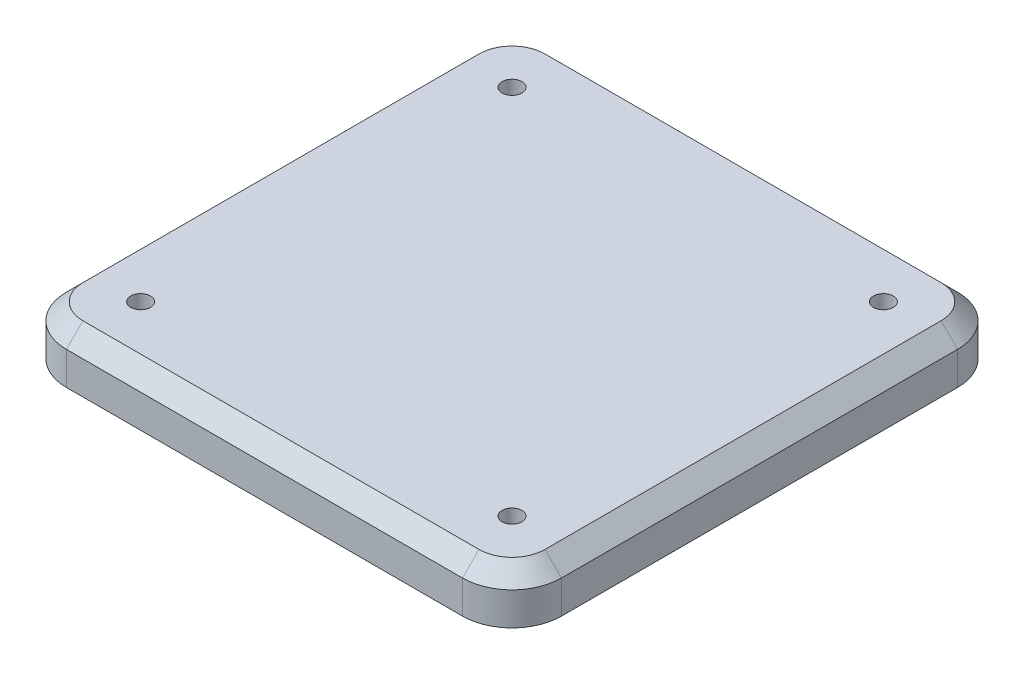
ISO-10303-21;
HEADER;
FILE_DESCRIPTION(('STEP AP214'),'2;1');
FILE_NAME('part.step','',(''),(''),'','','');
FILE_SCHEMA(('AUTOMOTIVE_DESIGN { 1 0 10303 214 1 1 1 1 }'));
ENDSEC;
DATA;
#1=APPLICATION_CONTEXT('core data for automotive mechanical design processes');
#2=APPLICATION_PROTOCOL_DEFINITION('international standard','automotive_design',2000,#1);
#3=PRODUCT_CONTEXT('',#1,'mechanical');
#4=PRODUCT('Part','Part','',(#3));
#5=PRODUCT_RELATED_PRODUCT_CATEGORY('part','',(#4));
#6=PRODUCT_DEFINITION_FORMATION('','',#4);
#7=PRODUCT_DEFINITION_CONTEXT('part definition',#1,'design');
#8=PRODUCT_DEFINITION('design','',#6,#7);
#9=PRODUCT_DEFINITION_SHAPE('','',#8);
#10=(LENGTH_UNIT() NAMED_UNIT(*) SI_UNIT(.MILLI.,.METRE.));
#11=(NAMED_UNIT(*) PLANE_ANGLE_UNIT() SI_UNIT($,.RADIAN.));
#12=(NAMED_UNIT(*) SI_UNIT($,.STERADIAN.) SOLID_ANGLE_UNIT());
#13=UNCERTAINTY_MEASURE_WITH_UNIT(LENGTH_MEASURE(1.E-05),#10,'distance_accuracy_value','');
#14=(GEOMETRIC_REPRESENTATION_CONTEXT(3) GLOBAL_UNCERTAINTY_ASSIGNED_CONTEXT((#13)) GLOBAL_UNIT_ASSIGNED_CONTEXT((#10,
#11,#12)) REPRESENTATION_CONTEXT('',''));
#15=CARTESIAN_POINT('',(0.,0.,0.));
#16=DIRECTION('',(0.,0.,1.));
#17=DIRECTION('',(1.,0.,0.));
#18=AXIS2_PLACEMENT_3D('',#15,#16,#17);
#19=CARTESIAN_POINT('',(150.,15.,150.));
#20=DIRECTION('',(-1.,0.,0.));
#21=DIRECTION('',(0.,0.,1.));
#22=AXIS2_PLACEMENT_3D('',#19,#20,#21);
#23=PLANE('',#22);
#24=DIRECTION('',(0.,-1.,0.));
#25=VECTOR('',#24,1.);
#26=CARTESIAN_POINT('',(150.,15.,-120.));
#27=LINE('',#26,#25);
#28=CARTESIAN_POINT('',(150.,-15.,-120.));
#29=VERTEX_POINT('',#28);
#30=CARTESIAN_POINT('',(150.,4.99999999999999,-120.));
#31=VERTEX_POINT('',#30);
#32=EDGE_CURVE('E245',#29,#31,#27,.F.);
#33=ORIENTED_EDGE('',*,*,#32,.T.);
#34=DIRECTION('',(0.,0.,1.));
#35=VECTOR('',#34,1.);
#36=CARTESIAN_POINT('',(150.,4.99999999999999,150.));
#37=LINE('',#36,#35);
#38=CARTESIAN_POINT('',(150.,4.99999999999999,120.));
#39=VERTEX_POINT('',#38);
#40=EDGE_CURVE('E11',#31,#39,#37,.T.);
#41=ORIENTED_EDGE('',*,*,#40,.T.);
#42=DIRECTION('',(0.,-1.,0.));
#43=VECTOR('',#42,1.);
#44=CARTESIAN_POINT('',(150.,15.,120.));
#45=LINE('',#44,#43);
#46=CARTESIAN_POINT('',(150.,-15.,120.));
#47=VERTEX_POINT('',#46);
#48=EDGE_CURVE('E242',#39,#47,#45,.T.);
#49=ORIENTED_EDGE('',*,*,#48,.T.);
#50=DIRECTION('',(0.,0.,-1.));
#51=VECTOR('',#50,1.);
#52=CARTESIAN_POINT('',(150.,-15.,150.));
#53=LINE('',#52,#51);
#54=EDGE_CURVE('E215',#47,#29,#53,.T.);
#55=ORIENTED_EDGE('',*,*,#54,.T.);
#56=EDGE_LOOP('',(#33,#41,#49,#55));
#57=FACE_BOUND('',#56,.T.);
#58=ADVANCED_FACE('F41',(#57),#23,.F.);
#59=CARTESIAN_POINT('',(-150.,15.,-150.));
#60=DIRECTION('',(0.,0.,1.));
#61=DIRECTION('',(1.,0.,0.));
#62=AXIS2_PLACEMENT_3D('',#59,#60,#61);
#63=PLANE('',#62);
#64=DIRECTION('',(0.,-1.,0.));
#65=VECTOR('',#64,1.);
#66=CARTESIAN_POINT('',(-120.,15.,-150.));
#67=LINE('',#66,#65);
#68=CARTESIAN_POINT('',(-120.,-15.,-150.));
#69=VERTEX_POINT('',#68);
#70=CARTESIAN_POINT('',(-120.,4.99999999999999,-150.));
#71=VERTEX_POINT('',#70);
#72=EDGE_CURVE('E247',#69,#71,#67,.F.);
#73=ORIENTED_EDGE('',*,*,#72,.T.);
#74=DIRECTION('',(1.,0.,0.));
#75=VECTOR('',#74,1.);
#76=CARTESIAN_POINT('',(-150.,4.99999999999999,-150.));
#77=LINE('',#76,#75);
#78=CARTESIAN_POINT('',(120.,4.99999999999999,-150.));
#79=VERTEX_POINT('',#78);
#80=EDGE_CURVE('E280',#71,#79,#77,.T.);
#81=ORIENTED_EDGE('',*,*,#80,.T.);
#82=DIRECTION('',(0.,-1.,0.));
#83=VECTOR('',#82,1.);
#84=CARTESIAN_POINT('',(120.,15.,-150.));
#85=LINE('',#84,#83);
#86=CARTESIAN_POINT('',(120.,-15.,-150.));
#87=VERTEX_POINT('',#86);
#88=EDGE_CURVE('E246',#79,#87,#85,.T.);
#89=ORIENTED_EDGE('',*,*,#88,.T.);
#90=DIRECTION('',(-1.,0.,0.));
#91=VECTOR('',#90,1.);
#92=CARTESIAN_POINT('',(-150.,-15.,-150.));
#93=LINE('',#92,#91);
#94=EDGE_CURVE('E213',#87,#69,#93,.T.);
#95=ORIENTED_EDGE('',*,*,#94,.T.);
#96=EDGE_LOOP('',(#73,#81,#89,#95));
#97=FACE_BOUND('',#96,.T.);
#98=ADVANCED_FACE('F335',(#97),#63,.F.);
#99=CARTESIAN_POINT('',(-150.,15.,150.));
#100=DIRECTION('',(1.,0.,0.));
#101=DIRECTION('',(0.,0.,-1.));
#102=AXIS2_PLACEMENT_3D('',#99,#100,#101);
#103=PLANE('',#102);
#104=DIRECTION('',(0.,-1.,0.));
#105=VECTOR('',#104,1.);
#106=CARTESIAN_POINT('',(-150.,15.,120.));
#107=LINE('',#106,#105);
#108=CARTESIAN_POINT('',(-150.,-15.,120.));
#109=VERTEX_POINT('',#108);
#110=CARTESIAN_POINT('',(-150.,4.99999999999999,120.));
#111=VERTEX_POINT('',#110);
#112=EDGE_CURVE('E237',#109,#111,#107,.F.);
#113=ORIENTED_EDGE('',*,*,#112,.T.);
#114=DIRECTION('',(0.,0.,-1.));
#115=VECTOR('',#114,1.);
#116=CARTESIAN_POINT('',(-150.,4.99999999999999,150.));
#117=LINE('',#116,#115);
#118=CARTESIAN_POINT('',(-150.,4.99999999999999,-120.));
#119=VERTEX_POINT('',#118);
#120=EDGE_CURVE('E267',#111,#119,#117,.T.);
#121=ORIENTED_EDGE('',*,*,#120,.T.);
#122=DIRECTION('',(0.,-1.,0.));
#123=VECTOR('',#122,1.);
#124=CARTESIAN_POINT('',(-150.,15.,-120.));
#125=LINE('',#124,#123);
#126=CARTESIAN_POINT('',(-150.,-15.,-120.));
#127=VERTEX_POINT('',#126);
#128=EDGE_CURVE('E240',#119,#127,#125,.T.);
#129=ORIENTED_EDGE('',*,*,#128,.T.);
#130=DIRECTION('',(0.,0.,1.));
#131=VECTOR('',#130,1.);
#132=CARTESIAN_POINT('',(-150.,-15.,150.));
#133=LINE('',#132,#131);
#134=EDGE_CURVE('E219',#127,#109,#133,.T.);
#135=ORIENTED_EDGE('',*,*,#134,.T.);
#136=EDGE_LOOP('',(#113,#121,#129,#135));
#137=FACE_BOUND('',#136,.T.);
#138=ADVANCED_FACE('F346',(#137),#103,.F.);
#139=CARTESIAN_POINT('',(-150.,15.,150.));
#140=DIRECTION('',(0.,0.,-1.));
#141=DIRECTION('',(-1.,0.,0.));
#142=AXIS2_PLACEMENT_3D('',#139,#140,#141);
#143=PLANE('',#142);
#144=DIRECTION('',(0.,-1.,0.));
#145=VECTOR('',#144,1.);
#146=CARTESIAN_POINT('',(120.,15.,150.));
#147=LINE('',#146,#145);
#148=CARTESIAN_POINT('',(120.,-15.,150.));
#149=VERTEX_POINT('',#148);
#150=CARTESIAN_POINT('',(120.,4.99999999999999,150.));
#151=VERTEX_POINT('',#150);
#152=EDGE_CURVE('E223',#149,#151,#147,.F.);
#153=ORIENTED_EDGE('',*,*,#152,.T.);
#154=DIRECTION('',(-1.,0.,0.));
#155=VECTOR('',#154,1.);
#156=CARTESIAN_POINT('',(-150.,4.99999999999999,150.));
#157=LINE('',#156,#155);
#158=CARTESIAN_POINT('',(-120.,4.99999999999999,150.));
#159=VERTEX_POINT('',#158);
#160=EDGE_CURVE('E273',#151,#159,#157,.T.);
#161=ORIENTED_EDGE('',*,*,#160,.T.);
#162=DIRECTION('',(0.,-1.,0.));
#163=VECTOR('',#162,1.);
#164=CARTESIAN_POINT('',(-120.,15.,150.));
#165=LINE('',#164,#163);
#166=CARTESIAN_POINT('',(-120.,-15.,150.));
#167=VERTEX_POINT('',#166);
#168=EDGE_CURVE('E227',#159,#167,#165,.T.);
#169=ORIENTED_EDGE('',*,*,#168,.T.);
#170=DIRECTION('',(1.,0.,0.));
#171=VECTOR('',#170,1.);
#172=CARTESIAN_POINT('',(-150.,-15.,150.));
#173=LINE('',#172,#171);
#174=EDGE_CURVE('E221',#167,#149,#173,.T.);
#175=ORIENTED_EDGE('',*,*,#174,.T.);
#176=EDGE_LOOP('',(#153,#161,#169,#175));
#177=FACE_BOUND('',#176,.T.);
#178=ADVANCED_FACE('F319',(#177),#143,.F.);
#179=CARTESIAN_POINT('',(0.,15.,0.));
#180=DIRECTION('',(0.,-1.,0.));
#181=DIRECTION('',(0.,0.,-1.));
#182=AXIS2_PLACEMENT_3D('',#179,#180,#181);
#183=PLANE('',#182);
#184=CARTESIAN_POINT('',(112.5,15.,-112.5));
#185=DIRECTION('',(0.,1.,0.));
#186=DIRECTION('',(0.,0.,1.));
#187=AXIS2_PLACEMENT_3D('',#184,#185,#186);
#188=CIRCLE('',#187,5.99999999999999);
#189=CARTESIAN_POINT('',(112.5,15.,-106.5));
#190=VERTEX_POINT('',#189);
#191=EDGE_CURVE('E190',#190,#190,#188,.T.);
#192=ORIENTED_EDGE('',*,*,#191,.F.);
#193=EDGE_LOOP('',(#192));
#194=FACE_BOUND('',#193,.T.);
#195=CARTESIAN_POINT('',(-112.5,15.,-112.5));
#196=DIRECTION('',(0.,1.,0.));
#197=DIRECTION('',(0.,0.,1.));
#198=AXIS2_PLACEMENT_3D('',#195,#196,#197);
#199=CIRCLE('',#198,5.99999999999999);
#200=CARTESIAN_POINT('',(-112.5,15.,-106.5));
#201=VERTEX_POINT('',#200);
#202=EDGE_CURVE('E194',#201,#201,#199,.T.);
#203=ORIENTED_EDGE('',*,*,#202,.F.);
#204=EDGE_LOOP('',(#203));
#205=FACE_BOUND('',#204,.T.);
#206=CARTESIAN_POINT('',(-112.5,15.,112.5));
#207=DIRECTION('',(0.,1.,0.));
#208=DIRECTION('',(0.,0.,1.));
#209=AXIS2_PLACEMENT_3D('',#206,#207,#208);
#210=CIRCLE('',#209,5.99999999999999);
#211=CARTESIAN_POINT('',(-112.5,15.,118.5));
#212=VERTEX_POINT('',#211);
#213=EDGE_CURVE('E198',#212,#212,#210,.T.);
#214=ORIENTED_EDGE('',*,*,#213,.F.);
#215=EDGE_LOOP('',(#214));
#216=FACE_BOUND('',#215,.T.);
#217=CARTESIAN_POINT('',(112.5,15.,112.5));
#218=DIRECTION('',(0.,1.,0.));
#219=DIRECTION('',(0.,0.,1.));
#220=AXIS2_PLACEMENT_3D('',#217,#218,#219);
#221=CIRCLE('',#220,5.99999999999999);
#222=CARTESIAN_POINT('',(112.5,15.,118.5));
#223=VERTEX_POINT('',#222);
#224=EDGE_CURVE('E204',#223,#223,#221,.T.);
#225=ORIENTED_EDGE('',*,*,#224,.F.);
#226=EDGE_LOOP('',(#225));
#227=FACE_BOUND('',#226,.T.);
#228=CARTESIAN_POINT('',(-120.,15.,-120.));
#229=DIRECTION('',(0.,-1.,0.));
#230=DIRECTION('',(0.,0.,-1.));
#231=AXIS2_PLACEMENT_3D('',#228,#229,#230);
#232=CIRCLE('',#231,20.);
#233=CARTESIAN_POINT('',(-120.,15.,-140.));
#234=VERTEX_POINT('',#233);
#235=CARTESIAN_POINT('',(-140.,15.,-120.));
#236=VERTEX_POINT('',#235);
#237=EDGE_CURVE('E261',#234,#236,#232,.F.);
#238=ORIENTED_EDGE('',*,*,#237,.T.);
#239=DIRECTION('',(0.,0.,1.));
#240=VECTOR('',#239,1.);
#241=CARTESIAN_POINT('',(-140.,15.,0.));
#242=LINE('',#241,#240);
#243=CARTESIAN_POINT('',(-140.,15.,120.));
#244=VERTEX_POINT('',#243);
#245=EDGE_CURVE('E265',#236,#244,#242,.T.);
#246=ORIENTED_EDGE('',*,*,#245,.T.);
#247=CARTESIAN_POINT('',(-120.,15.,120.));
#248=DIRECTION('',(0.,-1.,0.));
#249=DIRECTION('',(0.,0.,-1.));
#250=AXIS2_PLACEMENT_3D('',#247,#248,#249);
#251=CIRCLE('',#250,20.);
#252=CARTESIAN_POINT('',(-120.,15.,140.));
#253=VERTEX_POINT('',#252);
#254=EDGE_CURVE('E264',#244,#253,#251,.F.);
#255=ORIENTED_EDGE('',*,*,#254,.T.);
#256=DIRECTION('',(1.,0.,0.));
#257=VECTOR('',#256,1.);
#258=CARTESIAN_POINT('',(0.,15.,140.));
#259=LINE('',#258,#257);
#260=CARTESIAN_POINT('',(120.,15.,140.));
#261=VERTEX_POINT('',#260);
#262=EDGE_CURVE('E256',#253,#261,#259,.T.);
#263=ORIENTED_EDGE('',*,*,#262,.T.);
#264=CARTESIAN_POINT('',(120.,15.,120.));
#265=DIRECTION('',(0.,-1.,0.));
#266=DIRECTION('',(0.,0.,-1.));
#267=AXIS2_PLACEMENT_3D('',#264,#265,#266);
#268=CIRCLE('',#267,20.);
#269=CARTESIAN_POINT('',(140.,15.,120.));
#270=VERTEX_POINT('',#269);
#271=EDGE_CURVE('E253',#261,#270,#268,.F.);
#272=ORIENTED_EDGE('',*,*,#271,.T.);
#273=DIRECTION('',(0.,0.,-1.));
#274=VECTOR('',#273,1.);
#275=CARTESIAN_POINT('',(140.,15.,0.));
#276=LINE('',#275,#274);
#277=CARTESIAN_POINT('',(140.,15.,-120.));
#278=VERTEX_POINT('',#277);
#279=EDGE_CURVE('E252',#270,#278,#276,.T.);
#280=ORIENTED_EDGE('',*,*,#279,.T.);
#281=CARTESIAN_POINT('',(120.,15.,-120.));
#282=DIRECTION('',(0.,-1.,0.));
#283=DIRECTION('',(0.,0.,-1.));
#284=AXIS2_PLACEMENT_3D('',#281,#282,#283);
#285=CIRCLE('',#284,20.);
#286=CARTESIAN_POINT('',(120.,15.,-140.));
#287=VERTEX_POINT('',#286);
#288=EDGE_CURVE('E254',#278,#287,#285,.F.);
#289=ORIENTED_EDGE('',*,*,#288,.T.);
#290=DIRECTION('',(-1.,0.,0.));
#291=VECTOR('',#290,1.);
#292=CARTESIAN_POINT('',(0.,15.,-140.));
#293=LINE('',#292,#291);
#294=EDGE_CURVE('E260',#287,#234,#293,.T.);
#295=ORIENTED_EDGE('',*,*,#294,.T.);
#296=EDGE_LOOP('',(#238,#246,#255,#263,#272,#280,#289,#295));
#297=FACE_BOUND('',#296,.T.);
#298=ADVANCED_FACE('F356',(#194,#205,#216,#227,#297),#183,.F.);
#299=CARTESIAN_POINT('',(0.,-15.,0.));
#300=DIRECTION('',(0.,-1.,0.));
#301=DIRECTION('',(0.,0.,-1.));
#302=AXIS2_PLACEMENT_3D('',#299,#300,#301);
#303=PLANE('',#302);
#304=CARTESIAN_POINT('',(-125.,-15.,125.));
#305=DIRECTION('',(0.,-1.,0.));
#306=DIRECTION('',(0.,0.,-1.));
#307=AXIS2_PLACEMENT_3D('',#304,#305,#306);
#308=CIRCLE('',#307,5.99999999999999);
#309=CARTESIAN_POINT('',(-125.,-15.,119.));
#310=VERTEX_POINT('',#309);
#311=EDGE_CURVE('E164',#310,#310,#308,.T.);
#312=ORIENTED_EDGE('',*,*,#311,.F.);
#313=EDGE_LOOP('',(#312));
#314=FACE_BOUND('',#313,.T.);
#315=CARTESIAN_POINT('',(125.,-15.,125.));
#316=DIRECTION('',(0.,-1.,0.));
#317=DIRECTION('',(0.,0.,-1.));
#318=AXIS2_PLACEMENT_3D('',#315,#316,#317);
#319=CIRCLE('',#318,5.99999999999998);
#320=CARTESIAN_POINT('',(125.,-15.,119.));
#321=VERTEX_POINT('',#320);
#322=EDGE_CURVE('E165',#321,#321,#319,.T.);
#323=ORIENTED_EDGE('',*,*,#322,.F.);
#324=EDGE_LOOP('',(#323));
#325=FACE_BOUND('',#324,.T.);
#326=CARTESIAN_POINT('',(125.,-15.,-125.));
#327=DIRECTION('',(0.,-1.,0.));
#328=DIRECTION('',(0.,0.,-1.));
#329=AXIS2_PLACEMENT_3D('',#326,#327,#328);
#330=CIRCLE('',#329,5.99999999999998);
#331=CARTESIAN_POINT('',(125.,-15.,-131.));
#332=VERTEX_POINT('',#331);
#333=EDGE_CURVE('E174',#332,#332,#330,.T.);
#334=ORIENTED_EDGE('',*,*,#333,.F.);
#335=EDGE_LOOP('',(#334));
#336=FACE_BOUND('',#335,.T.);
#337=CARTESIAN_POINT('',(-125.,-15.,-125.));
#338=DIRECTION('',(0.,-1.,0.));
#339=DIRECTION('',(0.,0.,-1.));
#340=AXIS2_PLACEMENT_3D('',#337,#338,#339);
#341=CIRCLE('',#340,5.99999999999999);
#342=CARTESIAN_POINT('',(-125.,-15.,-131.));
#343=VERTEX_POINT('',#342);
#344=EDGE_CURVE('E181',#343,#343,#341,.T.);
#345=ORIENTED_EDGE('',*,*,#344,.F.);
#346=EDGE_LOOP('',(#345));
#347=FACE_BOUND('',#346,.T.);
#348=ORIENTED_EDGE('',*,*,#174,.F.);
#349=CARTESIAN_POINT('',(-120.,-15.,120.));
#350=DIRECTION('',(0.,-1.,0.));
#351=DIRECTION('',(0.,0.,-1.));
#352=AXIS2_PLACEMENT_3D('',#349,#350,#351);
#353=CIRCLE('',#352,30.);
#354=EDGE_CURVE('E232',#167,#109,#353,.T.);
#355=ORIENTED_EDGE('',*,*,#354,.T.);
#356=ORIENTED_EDGE('',*,*,#134,.F.);
#357=CARTESIAN_POINT('',(-120.,-15.,-120.));
#358=DIRECTION('',(0.,-1.,0.));
#359=DIRECTION('',(0.,0.,-1.));
#360=AXIS2_PLACEMENT_3D('',#357,#358,#359);
#361=CIRCLE('',#360,30.);
#362=EDGE_CURVE('E233',#127,#69,#361,.T.);
#363=ORIENTED_EDGE('',*,*,#362,.T.);
#364=ORIENTED_EDGE('',*,*,#94,.F.);
#365=CARTESIAN_POINT('',(120.,-15.,-120.));
#366=DIRECTION('',(0.,-1.,0.));
#367=DIRECTION('',(0.,0.,-1.));
#368=AXIS2_PLACEMENT_3D('',#365,#366,#367);
#369=CIRCLE('',#368,30.);
#370=EDGE_CURVE('E230',#87,#29,#369,.T.);
#371=ORIENTED_EDGE('',*,*,#370,.T.);
#372=ORIENTED_EDGE('',*,*,#54,.F.);
#373=CARTESIAN_POINT('',(120.,-15.,120.));
#374=DIRECTION('',(0.,-1.,0.));
#375=DIRECTION('',(0.,0.,-1.));
#376=AXIS2_PLACEMENT_3D('',#373,#374,#375);
#377=CIRCLE('',#376,30.);
#378=EDGE_CURVE('E231',#47,#149,#377,.T.);
#379=ORIENTED_EDGE('',*,*,#378,.T.);
#380=EDGE_LOOP('',(#348,#355,#356,#363,#364,#371,#372,#379));
#381=FACE_BOUND('',#380,.T.);
#382=ADVANCED_FACE('F324',(#314,#325,#336,#347,#381),#303,.T.);
#383=CARTESIAN_POINT('',(-120.,15.,120.));
#384=DIRECTION('',(0.,-1.,0.));
#385=DIRECTION('',(0.,0.,-1.));
#386=AXIS2_PLACEMENT_3D('',#383,#384,#385);
#387=CYLINDRICAL_SURFACE('',#386,30.);
#388=ORIENTED_EDGE('',*,*,#168,.F.);
#389=CARTESIAN_POINT('',(-120.,4.99999999999999,120.));
#390=DIRECTION('',(0.,-1.,0.));
#391=DIRECTION('',(0.,0.,-1.));
#392=AXIS2_PLACEMENT_3D('',#389,#390,#391);
#393=CIRCLE('',#392,30.);
#394=EDGE_CURVE('E272',#159,#111,#393,.T.);
#395=ORIENTED_EDGE('',*,*,#394,.T.);
#396=ORIENTED_EDGE('',*,*,#112,.F.);
#397=ORIENTED_EDGE('',*,*,#354,.F.);
#398=EDGE_LOOP('',(#388,#395,#396,#397));
#399=FACE_BOUND('',#398,.T.);
#400=ADVANCED_FACE('F382',(#399),#387,.T.);
#401=CARTESIAN_POINT('',(120.,15.,120.));
#402=DIRECTION('',(0.,-1.,0.));
#403=DIRECTION('',(0.,0.,-1.));
#404=AXIS2_PLACEMENT_3D('',#401,#402,#403);
#405=CYLINDRICAL_SURFACE('',#404,30.);
#406=ORIENTED_EDGE('',*,*,#48,.F.);
#407=CARTESIAN_POINT('',(120.,4.99999999999999,120.));
#408=DIRECTION('',(0.,-1.,0.));
#409=DIRECTION('',(0.,0.,-1.));
#410=AXIS2_PLACEMENT_3D('',#407,#408,#409);
#411=CIRCLE('',#410,30.);
#412=EDGE_CURVE('E276',#39,#151,#411,.T.);
#413=ORIENTED_EDGE('',*,*,#412,.T.);
#414=ORIENTED_EDGE('',*,*,#152,.F.);
#415=ORIENTED_EDGE('',*,*,#378,.F.);
#416=EDGE_LOOP('',(#406,#413,#414,#415));
#417=FACE_BOUND('',#416,.T.);
#418=ADVANCED_FACE('F314',(#417),#405,.T.);
#419=CARTESIAN_POINT('',(-120.,15.,-120.));
#420=DIRECTION('',(0.,-1.,0.));
#421=DIRECTION('',(0.,0.,-1.));
#422=AXIS2_PLACEMENT_3D('',#419,#420,#421);
#423=CYLINDRICAL_SURFACE('',#422,30.);
#424=ORIENTED_EDGE('',*,*,#128,.F.);
#425=CARTESIAN_POINT('',(-120.,4.99999999999999,-120.));
#426=DIRECTION('',(0.,-1.,0.));
#427=DIRECTION('',(0.,0.,-1.));
#428=AXIS2_PLACEMENT_3D('',#425,#426,#427);
#429=CIRCLE('',#428,30.);
#430=EDGE_CURVE('E271',#119,#71,#429,.T.);
#431=ORIENTED_EDGE('',*,*,#430,.T.);
#432=ORIENTED_EDGE('',*,*,#72,.F.);
#433=ORIENTED_EDGE('',*,*,#362,.F.);
#434=EDGE_LOOP('',(#424,#431,#432,#433));
#435=FACE_BOUND('',#434,.T.);
#436=ADVANCED_FACE('F337',(#435),#423,.T.);
#437=CARTESIAN_POINT('',(120.,15.,-120.));
#438=DIRECTION('',(0.,-1.,0.));
#439=DIRECTION('',(0.,0.,-1.));
#440=AXIS2_PLACEMENT_3D('',#437,#438,#439);
#441=CYLINDRICAL_SURFACE('',#440,30.);
#442=ORIENTED_EDGE('',*,*,#88,.F.);
#443=CARTESIAN_POINT('',(120.,4.99999999999999,-120.));
#444=DIRECTION('',(0.,-1.,0.));
#445=DIRECTION('',(0.,0.,-1.));
#446=AXIS2_PLACEMENT_3D('',#443,#444,#445);
#447=CIRCLE('',#446,30.);
#448=EDGE_CURVE('E51',#79,#31,#447,.T.);
#449=ORIENTED_EDGE('',*,*,#448,.T.);
#450=ORIENTED_EDGE('',*,*,#32,.F.);
#451=ORIENTED_EDGE('',*,*,#370,.F.);
#452=EDGE_LOOP('',(#442,#449,#450,#451));
#453=FACE_BOUND('',#452,.T.);
#454=ADVANCED_FACE('F329',(#453),#441,.T.);
#455=CARTESIAN_POINT('',(140.,15.,0.));
#456=DIRECTION('',(-0.707106781186547,-0.707106781186547,0.));
#457=DIRECTION('',(0.,0.,-1.));
#458=AXIS2_PLACEMENT_3D('',#455,#456,#457);
#459=PLANE('',#458);
#460=DIRECTION('',(-0.707106781186547,0.707106781186547,0.));
#461=VECTOR('',#460,1.);
#462=CARTESIAN_POINT('',(150.,4.99999999999999,120.));
#463=LINE('',#462,#461);
#464=EDGE_CURVE('E298',#39,#270,#463,.T.);
#465=ORIENTED_EDGE('',*,*,#464,.F.);
#466=ORIENTED_EDGE('',*,*,#40,.F.);
#467=DIRECTION('',(0.707106781186547,-0.707106781186547,0.));
#468=VECTOR('',#467,1.);
#469=CARTESIAN_POINT('',(140.,15.,-120.));
#470=LINE('',#469,#468);
#471=EDGE_CURVE('E46',#278,#31,#470,.T.);
#472=ORIENTED_EDGE('',*,*,#471,.F.);
#473=ORIENTED_EDGE('',*,*,#279,.F.);
#474=EDGE_LOOP('',(#465,#466,#472,#473));
#475=FACE_BOUND('',#474,.T.);
#476=ADVANCED_FACE('F42',(#475),#459,.F.);
#477=CARTESIAN_POINT('',(120.,15.,-120.));
#478=DIRECTION('',(0.,-1.,0.));
#479=DIRECTION('',(0.,0.,-1.));
#480=AXIS2_PLACEMENT_3D('',#477,#478,#479);
#481=CONICAL_SURFACE('',#480,20.,0.785398163397448);
#482=ORIENTED_EDGE('',*,*,#471,.T.);
#483=ORIENTED_EDGE('',*,*,#448,.F.);
#484=DIRECTION('',(0.,-0.707106781186547,-0.707106781186547));
#485=VECTOR('',#484,1.);
#486=CARTESIAN_POINT('',(120.,15.,-140.));
#487=LINE('',#486,#485);
#488=EDGE_CURVE('E295',#287,#79,#487,.T.);
#489=ORIENTED_EDGE('',*,*,#488,.F.);
#490=ORIENTED_EDGE('',*,*,#288,.F.);
#491=EDGE_LOOP('',(#482,#483,#489,#490));
#492=FACE_BOUND('',#491,.T.);
#493=ADVANCED_FACE('F306',(#492),#481,.T.);
#494=CARTESIAN_POINT('',(120.,15.,120.));
#495=DIRECTION('',(0.,-1.,0.));
#496=DIRECTION('',(0.,0.,-1.));
#497=AXIS2_PLACEMENT_3D('',#494,#495,#496);
#498=CONICAL_SURFACE('',#497,20.,0.785398163397448);
#499=ORIENTED_EDGE('',*,*,#464,.T.);
#500=ORIENTED_EDGE('',*,*,#271,.F.);
#501=DIRECTION('',(0.,0.707106781186547,-0.707106781186547));
#502=VECTOR('',#501,1.);
#503=CARTESIAN_POINT('',(120.,4.99999999999999,150.));
#504=LINE('',#503,#502);
#505=EDGE_CURVE('E293',#151,#261,#504,.T.);
#506=ORIENTED_EDGE('',*,*,#505,.F.);
#507=ORIENTED_EDGE('',*,*,#412,.F.);
#508=EDGE_LOOP('',(#499,#500,#506,#507));
#509=FACE_BOUND('',#508,.T.);
#510=ADVANCED_FACE('F311',(#509),#498,.T.);
#511=CARTESIAN_POINT('',(0.,15.,-140.));
#512=DIRECTION('',(0.,-0.707106781186547,0.707106781186547));
#513=DIRECTION('',(-1.,0.,0.));
#514=AXIS2_PLACEMENT_3D('',#511,#512,#513);
#515=PLANE('',#514);
#516=ORIENTED_EDGE('',*,*,#488,.T.);
#517=ORIENTED_EDGE('',*,*,#80,.F.);
#518=DIRECTION('',(0.,-0.707106781186547,-0.707106781186547));
#519=VECTOR('',#518,1.);
#520=CARTESIAN_POINT('',(-120.,15.,-140.));
#521=LINE('',#520,#519);
#522=EDGE_CURVE('E287',#234,#71,#521,.T.);
#523=ORIENTED_EDGE('',*,*,#522,.F.);
#524=ORIENTED_EDGE('',*,*,#294,.F.);
#525=EDGE_LOOP('',(#516,#517,#523,#524));
#526=FACE_BOUND('',#525,.T.);
#527=ADVANCED_FACE('F363',(#526),#515,.F.);
#528=CARTESIAN_POINT('',(0.,15.,140.));
#529=DIRECTION('',(0.,-0.707106781186547,-0.707106781186547));
#530=DIRECTION('',(1.,0.,0.));
#531=AXIS2_PLACEMENT_3D('',#528,#529,#530);
#532=PLANE('',#531);
#533=ORIENTED_EDGE('',*,*,#505,.T.);
#534=ORIENTED_EDGE('',*,*,#262,.F.);
#535=DIRECTION('',(0.,0.707106781186547,-0.707106781186547));
#536=VECTOR('',#535,1.);
#537=CARTESIAN_POINT('',(-120.,4.99999999999999,150.));
#538=LINE('',#537,#536);
#539=EDGE_CURVE('E285',#159,#253,#538,.T.);
#540=ORIENTED_EDGE('',*,*,#539,.F.);
#541=ORIENTED_EDGE('',*,*,#160,.F.);
#542=EDGE_LOOP('',(#533,#534,#540,#541));
#543=FACE_BOUND('',#542,.T.);
#544=ADVANCED_FACE('F361',(#543),#532,.F.);
#545=CARTESIAN_POINT('',(-120.,15.,-120.));
#546=DIRECTION('',(0.,-1.,0.));
#547=DIRECTION('',(0.,0.,-1.));
#548=AXIS2_PLACEMENT_3D('',#545,#546,#547);
#549=CONICAL_SURFACE('',#548,20.,0.785398163397448);
#550=ORIENTED_EDGE('',*,*,#522,.T.);
#551=ORIENTED_EDGE('',*,*,#430,.F.);
#552=DIRECTION('',(-0.707106781186547,-0.707106781186547,0.));
#553=VECTOR('',#552,1.);
#554=CARTESIAN_POINT('',(-140.,15.,-120.));
#555=LINE('',#554,#553);
#556=EDGE_CURVE('E284',#236,#119,#555,.T.);
#557=ORIENTED_EDGE('',*,*,#556,.F.);
#558=ORIENTED_EDGE('',*,*,#237,.F.);
#559=EDGE_LOOP('',(#550,#551,#557,#558));
#560=FACE_BOUND('',#559,.T.);
#561=ADVANCED_FACE('F338',(#560),#549,.T.);
#562=CARTESIAN_POINT('',(-120.,15.,120.));
#563=DIRECTION('',(0.,-1.,0.));
#564=DIRECTION('',(0.,0.,-1.));
#565=AXIS2_PLACEMENT_3D('',#562,#563,#564);
#566=CONICAL_SURFACE('',#565,20.,0.785398163397448);
#567=ORIENTED_EDGE('',*,*,#539,.T.);
#568=ORIENTED_EDGE('',*,*,#254,.F.);
#569=DIRECTION('',(0.707106781186547,0.707106781186547,0.));
#570=VECTOR('',#569,1.);
#571=CARTESIAN_POINT('',(-150.,4.99999999999999,120.));
#572=LINE('',#571,#570);
#573=EDGE_CURVE('E212',#111,#244,#572,.T.);
#574=ORIENTED_EDGE('',*,*,#573,.F.);
#575=ORIENTED_EDGE('',*,*,#394,.F.);
#576=EDGE_LOOP('',(#567,#568,#574,#575));
#577=FACE_BOUND('',#576,.T.);
#578=ADVANCED_FACE('F353',(#577),#566,.T.);
#579=CARTESIAN_POINT('',(-140.,15.,0.));
#580=DIRECTION('',(0.707106781186547,-0.707106781186547,0.));
#581=DIRECTION('',(0.,0.,1.));
#582=AXIS2_PLACEMENT_3D('',#579,#580,#581);
#583=PLANE('',#582);
#584=ORIENTED_EDGE('',*,*,#556,.T.);
#585=ORIENTED_EDGE('',*,*,#120,.F.);
#586=ORIENTED_EDGE('',*,*,#573,.T.);
#587=ORIENTED_EDGE('',*,*,#245,.F.);
#588=EDGE_LOOP('',(#584,#585,#586,#587));
#589=FACE_BOUND('',#588,.T.);
#590=ADVANCED_FACE('F350',(#589),#583,.F.);
#591=CARTESIAN_POINT('',(112.5,5.,112.5));
#592=DIRECTION('',(0.,1.,0.));
#593=DIRECTION('',(0.,0.,1.));
#594=AXIS2_PLACEMENT_3D('',#591,#592,#593);
#595=CONICAL_SURFACE('',#594,5.99999999999999,1.02974425867665);
#596=CARTESIAN_POINT('',(112.5,1.39483628583464,112.5));
#597=VERTEX_POINT('',#596);
#598=VERTEX_LOOP('',#597);
#599=FACE_BOUND('',#598,.T.);
#600=CARTESIAN_POINT('',(112.5,5.,112.5));
#601=DIRECTION('',(0.,1.,0.));
#602=DIRECTION('',(0.,0.,1.));
#603=AXIS2_PLACEMENT_3D('',#600,#601,#602);
#604=CIRCLE('',#603,5.99999999999999);
#605=CARTESIAN_POINT('',(112.5,5.,118.5));
#606=VERTEX_POINT('',#605);
#607=EDGE_CURVE('E206',#606,#606,#604,.T.);
#608=ORIENTED_EDGE('',*,*,#607,.T.);
#609=EDGE_LOOP('',(#608));
#610=FACE_BOUND('',#609,.T.);
#611=ADVANCED_FACE('F400',(#599,#610),#595,.F.);
#612=CARTESIAN_POINT('',(112.5,15.,112.5));
#613=DIRECTION('',(0.,1.,0.));
#614=DIRECTION('',(0.,0.,1.));
#615=AXIS2_PLACEMENT_3D('',#612,#613,#614);
#616=CYLINDRICAL_SURFACE('',#615,5.99999999999999);
#617=ORIENTED_EDGE('',*,*,#607,.F.);
#618=EDGE_LOOP('',(#617));
#619=FACE_BOUND('',#618,.T.);
#620=ORIENTED_EDGE('',*,*,#224,.T.);
#621=EDGE_LOOP('',(#620));
#622=FACE_BOUND('',#621,.T.);
#623=ADVANCED_FACE('F535',(#619,#622),#616,.F.);
#624=CARTESIAN_POINT('',(-112.5,5.,112.5));
#625=DIRECTION('',(0.,1.,0.));
#626=DIRECTION('',(0.,0.,1.));
#627=AXIS2_PLACEMENT_3D('',#624,#625,#626);
#628=CONICAL_SURFACE('',#627,5.99999999999999,1.02974425867665);
#629=CARTESIAN_POINT('',(-112.5,1.39483628583464,112.5));
#630=VERTEX_POINT('',#629);
#631=VERTEX_LOOP('',#630);
#632=FACE_BOUND('',#631,.T.);
#633=CARTESIAN_POINT('',(-112.5,5.,112.5));
#634=DIRECTION('',(0.,1.,0.));
#635=DIRECTION('',(0.,0.,1.));
#636=AXIS2_PLACEMENT_3D('',#633,#634,#635);
#637=CIRCLE('',#636,5.99999999999999);
#638=CARTESIAN_POINT('',(-112.5,5.,118.5));
#639=VERTEX_POINT('',#638);
#640=EDGE_CURVE('E205',#639,#639,#637,.T.);
#641=ORIENTED_EDGE('',*,*,#640,.T.);
#642=EDGE_LOOP('',(#641));
#643=FACE_BOUND('',#642,.T.);
#644=ADVANCED_FACE('F541',(#632,#643),#628,.F.);
#645=CARTESIAN_POINT('',(-112.5,15.,112.5));
#646=DIRECTION('',(0.,1.,0.));
#647=DIRECTION('',(0.,0.,1.));
#648=AXIS2_PLACEMENT_3D('',#645,#646,#647);
#649=CYLINDRICAL_SURFACE('',#648,5.99999999999999);
#650=ORIENTED_EDGE('',*,*,#640,.F.);
#651=EDGE_LOOP('',(#650));
#652=FACE_BOUND('',#651,.T.);
#653=ORIENTED_EDGE('',*,*,#213,.T.);
#654=EDGE_LOOP('',(#653));
#655=FACE_BOUND('',#654,.T.);
#656=ADVANCED_FACE('F549',(#652,#655),#649,.F.);
#657=CARTESIAN_POINT('',(-112.5,5.,-112.5));
#658=DIRECTION('',(0.,1.,0.));
#659=DIRECTION('',(0.,0.,1.));
#660=AXIS2_PLACEMENT_3D('',#657,#658,#659);
#661=CONICAL_SURFACE('',#660,5.99999999999999,1.02974425867665);
#662=CARTESIAN_POINT('',(-112.5,1.39483628583464,-112.5));
#663=VERTEX_POINT('',#662);
#664=VERTEX_LOOP('',#663);
#665=FACE_BOUND('',#664,.T.);
#666=CARTESIAN_POINT('',(-112.5,5.,-112.5));
#667=DIRECTION('',(0.,1.,0.));
#668=DIRECTION('',(0.,0.,1.));
#669=AXIS2_PLACEMENT_3D('',#666,#667,#668);
#670=CIRCLE('',#669,5.99999999999999);
#671=CARTESIAN_POINT('',(-112.5,5.,-106.5));
#672=VERTEX_POINT('',#671);
#673=EDGE_CURVE('E196',#672,#672,#670,.T.);
#674=ORIENTED_EDGE('',*,*,#673,.T.);
#675=EDGE_LOOP('',(#674));
#676=FACE_BOUND('',#675,.T.);
#677=ADVANCED_FACE('F559',(#665,#676),#661,.F.);
#678=CARTESIAN_POINT('',(-112.5,15.,-112.5));
#679=DIRECTION('',(0.,1.,0.));
#680=DIRECTION('',(0.,0.,1.));
#681=AXIS2_PLACEMENT_3D('',#678,#679,#680);
#682=CYLINDRICAL_SURFACE('',#681,5.99999999999999);
#683=ORIENTED_EDGE('',*,*,#673,.F.);
#684=EDGE_LOOP('',(#683));
#685=FACE_BOUND('',#684,.T.);
#686=ORIENTED_EDGE('',*,*,#202,.T.);
#687=EDGE_LOOP('',(#686));
#688=FACE_BOUND('',#687,.T.);
#689=ADVANCED_FACE('F568',(#685,#688),#682,.F.);
#690=CARTESIAN_POINT('',(112.5,5.,-112.5));
#691=DIRECTION('',(0.,1.,0.));
#692=DIRECTION('',(0.,0.,1.));
#693=AXIS2_PLACEMENT_3D('',#690,#691,#692);
#694=CONICAL_SURFACE('',#693,5.99999999999999,1.02974425867665);
#695=CARTESIAN_POINT('',(112.5,1.39483628583464,-112.5));
#696=VERTEX_POINT('',#695);
#697=VERTEX_LOOP('',#696);
#698=FACE_BOUND('',#697,.T.);
#699=CARTESIAN_POINT('',(112.5,5.,-112.5));
#700=DIRECTION('',(0.,1.,0.));
#701=DIRECTION('',(0.,0.,1.));
#702=AXIS2_PLACEMENT_3D('',#699,#700,#701);
#703=CIRCLE('',#702,5.99999999999999);
#704=CARTESIAN_POINT('',(112.5,5.,-106.5));
#705=VERTEX_POINT('',#704);
#706=EDGE_CURVE('E188',#705,#705,#703,.T.);
#707=ORIENTED_EDGE('',*,*,#706,.T.);
#708=EDGE_LOOP('',(#707));
#709=FACE_BOUND('',#708,.T.);
#710=ADVANCED_FACE('F580',(#698,#709),#694,.F.);
#711=CARTESIAN_POINT('',(112.5,15.,-112.5));
#712=DIRECTION('',(0.,1.,0.));
#713=DIRECTION('',(0.,0.,1.));
#714=AXIS2_PLACEMENT_3D('',#711,#712,#713);
#715=CYLINDRICAL_SURFACE('',#714,5.99999999999999);
#716=ORIENTED_EDGE('',*,*,#706,.F.);
#717=EDGE_LOOP('',(#716));
#718=FACE_BOUND('',#717,.T.);
#719=ORIENTED_EDGE('',*,*,#191,.T.);
#720=EDGE_LOOP('',(#719));
#721=FACE_BOUND('',#720,.T.);
#722=ADVANCED_FACE('F586',(#718,#721),#715,.F.);
#723=CARTESIAN_POINT('',(-125.,-5.,-125.));
#724=DIRECTION('',(0.,-1.,0.));
#725=DIRECTION('',(0.,0.,-1.));
#726=AXIS2_PLACEMENT_3D('',#723,#724,#725);
#727=CONICAL_SURFACE('',#726,5.99999999999999,1.02974425867665);
#728=CARTESIAN_POINT('',(-125.,-1.39483628583464,-125.));
#729=VERTEX_POINT('',#728);
#730=VERTEX_LOOP('',#729);
#731=FACE_BOUND('',#730,.T.);
#732=CARTESIAN_POINT('',(-125.,-5.,-125.));
#733=DIRECTION('',(0.,-1.,0.));
#734=DIRECTION('',(0.,0.,-1.));
#735=AXIS2_PLACEMENT_3D('',#732,#733,#734);
#736=CIRCLE('',#735,5.99999999999999);
#737=CARTESIAN_POINT('',(-125.,-5.,-131.));
#738=VERTEX_POINT('',#737);
#739=EDGE_CURVE('E183',#738,#738,#736,.T.);
#740=ORIENTED_EDGE('',*,*,#739,.T.);
#741=EDGE_LOOP('',(#740));
#742=FACE_BOUND('',#741,.T.);
#743=ADVANCED_FACE('F594',(#731,#742),#727,.F.);
#744=CARTESIAN_POINT('',(-125.,-15.,-125.));
#745=DIRECTION('',(0.,-1.,0.));
#746=DIRECTION('',(0.,0.,-1.));
#747=AXIS2_PLACEMENT_3D('',#744,#745,#746);
#748=CYLINDRICAL_SURFACE('',#747,5.99999999999999);
#749=ORIENTED_EDGE('',*,*,#739,.F.);
#750=EDGE_LOOP('',(#749));
#751=FACE_BOUND('',#750,.T.);
#752=ORIENTED_EDGE('',*,*,#344,.T.);
#753=EDGE_LOOP('',(#752));
#754=FACE_BOUND('',#753,.T.);
#755=ADVANCED_FACE('F601',(#751,#754),#748,.F.);
#756=CARTESIAN_POINT('',(125.,-5.,-125.));
#757=DIRECTION('',(0.,-1.,0.));
#758=DIRECTION('',(0.,0.,-1.));
#759=AXIS2_PLACEMENT_3D('',#756,#757,#758);
#760=CONICAL_SURFACE('',#759,5.99999999999998,1.02974425867665);
#761=CARTESIAN_POINT('',(125.,-1.39483628583464,-125.));
#762=VERTEX_POINT('',#761);
#763=VERTEX_LOOP('',#762);
#764=FACE_BOUND('',#763,.T.);
#765=CARTESIAN_POINT('',(125.,-5.,-125.));
#766=DIRECTION('',(0.,-1.,0.));
#767=DIRECTION('',(0.,0.,-1.));
#768=AXIS2_PLACEMENT_3D('',#765,#766,#767);
#769=CIRCLE('',#768,5.99999999999998);
#770=CARTESIAN_POINT('',(125.,-5.,-131.));
#771=VERTEX_POINT('',#770);
#772=EDGE_CURVE('E178',#771,#771,#769,.T.);
#773=ORIENTED_EDGE('',*,*,#772,.T.);
#774=EDGE_LOOP('',(#773));
#775=FACE_BOUND('',#774,.T.);
#776=ADVANCED_FACE('F612',(#764,#775),#760,.F.);
#777=CARTESIAN_POINT('',(125.,-15.,-125.));
#778=DIRECTION('',(0.,-1.,0.));
#779=DIRECTION('',(0.,0.,-1.));
#780=AXIS2_PLACEMENT_3D('',#777,#778,#779);
#781=CYLINDRICAL_SURFACE('',#780,5.99999999999998);
#782=ORIENTED_EDGE('',*,*,#772,.F.);
#783=EDGE_LOOP('',(#782));
#784=FACE_BOUND('',#783,.T.);
#785=ORIENTED_EDGE('',*,*,#333,.T.);
#786=EDGE_LOOP('',(#785));
#787=FACE_BOUND('',#786,.T.);
#788=ADVANCED_FACE('F625',(#784,#787),#781,.F.);
#789=CARTESIAN_POINT('',(125.,-5.,125.));
#790=DIRECTION('',(0.,-1.,0.));
#791=DIRECTION('',(0.,0.,-1.));
#792=AXIS2_PLACEMENT_3D('',#789,#790,#791);
#793=CONICAL_SURFACE('',#792,5.99999999999998,1.02974425867665);
#794=CARTESIAN_POINT('',(125.,-1.39483628583464,125.));
#795=VERTEX_POINT('',#794);
#796=VERTEX_LOOP('',#795);
#797=FACE_BOUND('',#796,.T.);
#798=CARTESIAN_POINT('',(125.,-5.,125.));
#799=DIRECTION('',(0.,-1.,0.));
#800=DIRECTION('',(0.,0.,-1.));
#801=AXIS2_PLACEMENT_3D('',#798,#799,#800);
#802=CIRCLE('',#801,5.99999999999998);
#803=CARTESIAN_POINT('',(125.,-5.,119.));
#804=VERTEX_POINT('',#803);
#805=EDGE_CURVE('E166',#804,#804,#802,.T.);
#806=ORIENTED_EDGE('',*,*,#805,.T.);
#807=EDGE_LOOP('',(#806));
#808=FACE_BOUND('',#807,.T.);
#809=ADVANCED_FACE('F631',(#797,#808),#793,.F.);
#810=CARTESIAN_POINT('',(125.,-15.,125.));
#811=DIRECTION('',(0.,-1.,0.));
#812=DIRECTION('',(0.,0.,-1.));
#813=AXIS2_PLACEMENT_3D('',#810,#811,#812);
#814=CYLINDRICAL_SURFACE('',#813,5.99999999999998);
#815=ORIENTED_EDGE('',*,*,#805,.F.);
#816=EDGE_LOOP('',(#815));
#817=FACE_BOUND('',#816,.T.);
#818=ORIENTED_EDGE('',*,*,#322,.T.);
#819=EDGE_LOOP('',(#818));
#820=FACE_BOUND('',#819,.T.);
#821=ADVANCED_FACE('F157',(#817,#820),#814,.F.);
#822=CARTESIAN_POINT('',(-125.,-5.,125.));
#823=DIRECTION('',(0.,-1.,0.));
#824=DIRECTION('',(0.,0.,-1.));
#825=AXIS2_PLACEMENT_3D('',#822,#823,#824);
#826=CONICAL_SURFACE('',#825,5.99999999999999,1.02974425867665);
#827=CARTESIAN_POINT('',(-125.,-1.39483628583464,125.));
#828=VERTEX_POINT('',#827);
#829=VERTEX_LOOP('',#828);
#830=FACE_BOUND('',#829,.T.);
#831=CARTESIAN_POINT('',(-125.,-5.,125.));
#832=DIRECTION('',(0.,-1.,0.));
#833=DIRECTION('',(0.,0.,-1.));
#834=AXIS2_PLACEMENT_3D('',#831,#832,#833);
#835=CIRCLE('',#834,5.99999999999999);
#836=CARTESIAN_POINT('',(-125.,-5.,119.));
#837=VERTEX_POINT('',#836);
#838=EDGE_CURVE('E162',#837,#837,#835,.T.);
#839=ORIENTED_EDGE('',*,*,#838,.T.);
#840=EDGE_LOOP('',(#839));
#841=FACE_BOUND('',#840,.T.);
#842=ADVANCED_FACE('F153',(#830,#841),#826,.F.);
#843=CARTESIAN_POINT('',(-125.,-15.,125.));
#844=DIRECTION('',(0.,-1.,0.));
#845=DIRECTION('',(0.,0.,-1.));
#846=AXIS2_PLACEMENT_3D('',#843,#844,#845);
#847=CYLINDRICAL_SURFACE('',#846,5.99999999999999);
#848=ORIENTED_EDGE('',*,*,#838,.F.);
#849=EDGE_LOOP('',(#848));
#850=FACE_BOUND('',#849,.T.);
#851=ORIENTED_EDGE('',*,*,#311,.T.);
#852=EDGE_LOOP('',(#851));
#853=FACE_BOUND('',#852,.T.);
#854=ADVANCED_FACE('F160',(#850,#853),#847,.F.);
#855=CLOSED_SHELL('',(#58,#98,#138,#178,#298,#382,#400,#418,#436,#454,#476,#493,#510,#527,#544,
#561,#578,#590,#611,#623,#644,#656,#677,#689,#710,#722,#743,#755,#776,#788,#809,#821,#842,#854));
#856=MANIFOLD_SOLID_BREP('B2',#855);
#857=ADVANCED_BREP_SHAPE_REPRESENTATION('',(#18,#856),#14);
#858=SHAPE_DEFINITION_REPRESENTATION(#9,#857);
ENDSEC;
END-ISO-10303-21;
